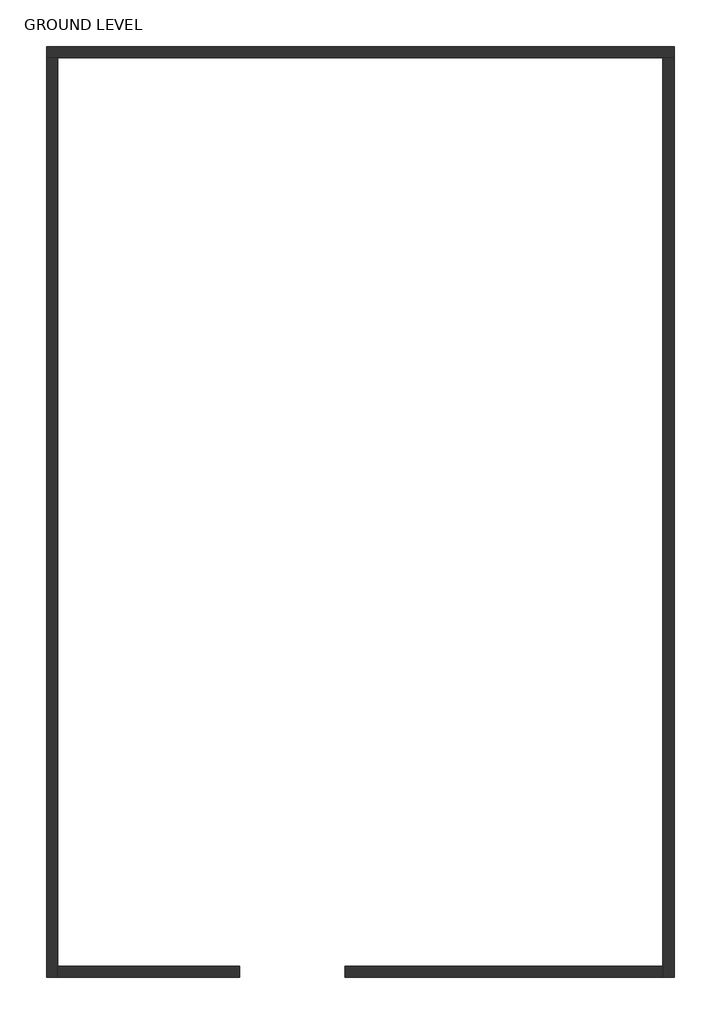
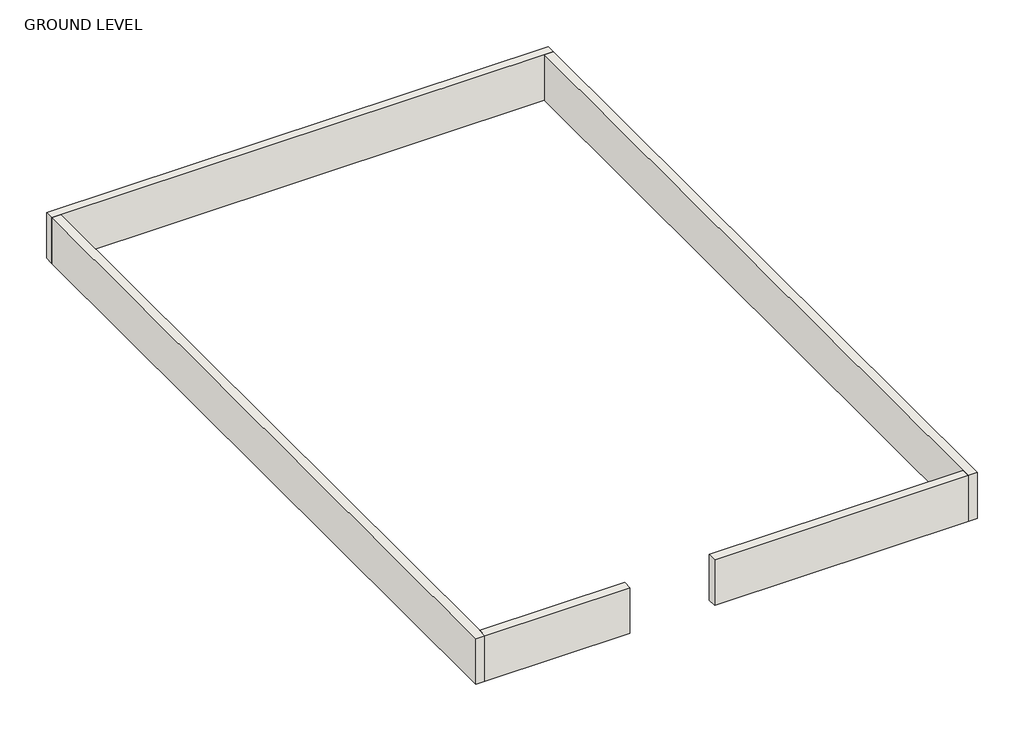
# One storey: 5 walls.
"""IFC4 building model written with IfcOpenShell, lengths in millimetres."""

from ifc_helpers import new_model, si_unit, origin, origin_with_axes, place, context, project, spatial, polyline, outline, extrude, faceted_brep, element, save

model = new_model("IFC4")

# Units and contexts
model_context = context("Model", 3, world=origin())
ifc_project = project(units=[si_unit("LENGTHUNIT", "METRE", prefix="MILLI")], contexts=[model_context])

# Site, building, storey
site = spatial("IfcSite", under=ifc_project)
building = spatial("IfcBuilding", under=site)
storey = spatial("IfcBuildingStorey", under=building, Name="GROUND LEVEL", Elevation=0.0)

# Walls
placement = place(None, origin())
element("IfcWall", 1, ObjectType="EXTERIOR WALL 9\"", at=placement, inside=storey, context=model_context, shape_type="Brep", body=[
    faceted_brep([(-19973.9229553, 9244.8839313, 0.0), (-19745.3229553, 9244.8839313, 0.0), (-7553.3229553, 9244.8839313, 0.0), (-7324.7229553, 9244.8839313, 0.0), (-7324.7229553, 9244.8839313, 1219.2), (-7553.3229553, 9244.8839313, 1219.2), (-19745.3229553, 9244.8839313, 1219.2), (-19973.9229553, 9244.8839313, 1219.2), (-19973.9229553, 9473.4839313, 0.0), (-19973.9229553, 9473.4839313, 1219.2), (-7324.7229553, 9473.4839313, 1219.2), (-7324.7229553, 9473.4839313, 0.0)], [[[0, 1, 2, 3, 4, 5, 6, 7]], [[8, 9, 10, 11]], [[3, 2, 1, 0, 8, 11]], [[7, 6, 5, 4, 10, 9]], [[4, 3, 11, 10]], [[0, 7, 9, 8]]]),
])
element("IfcWall", 2, ObjectType="EXTERIOR WALL 9\"", at=placement, inside=storey, context=model_context, shape_type="Brep", body=[
    faceted_brep([(-7553.3229553, 9244.8839313, 0.0), (-7553.3229553, -9044.7035687, 0.0), (-7553.3229553, -9273.3035687, 0.0), (-7553.3229553, -9273.3035687, 1219.2), (-7553.3229553, -9044.7035687, 1219.2), (-7553.3229553, 9244.8839313, 1219.2), (-7324.7229553, 9244.8839313, 0.0), (-7324.7229553, 9244.8839313, 1219.2), (-7324.7229553, -9273.3035687, 1219.2), (-7324.7229553, -9273.3035687, 0.0)], [[[0, 1, 2, 3, 4, 5]], [[6, 7, 8, 9]], [[2, 1, 0, 6, 9]], [[5, 4, 3, 8, 7]], [[0, 5, 7, 6]], [[3, 2, 9, 8]]]),
])
element("IfcWall", 3, ObjectType="EXTERIOR WALL 9\"", at=placement, inside=storey, context=model_context, shape_type="SweptSolid", body=[
    extrude(outline(polyline([(-13954.1229553, -9044.7035687), (-7553.3229553, -9044.7035687), (-7553.3229553, -9273.3035687), (-13954.1229553, -9273.3035687), (-13954.1229553, -9044.7035687)])), origin_with_axes(), (0.0, 0.0, 1.0), 1219.2),
])
element("IfcWall", 4, ObjectType="EXTERIOR WALL 9\"", at=placement, inside=storey, context=model_context, shape_type="Brep", body=[
    faceted_brep([(-19745.3229553, -9273.3035687, 0.0), (-19745.3229553, -9044.7035687, 0.0), (-19745.3229553, 9244.8839313, 0.0), (-19745.3229553, 9244.8839313, 1219.2), (-19745.3229553, -9044.7035687, 1219.2), (-19745.3229553, -9273.3035687, 1219.2), (-19973.9229553, -9273.3035687, 0.0), (-19973.9229553, -9273.3035687, 1219.2), (-19973.9229553, 9244.8839313, 1219.2), (-19973.9229553, 9244.8839313, 0.0)], [[[0, 1, 2, 3, 4, 5]], [[6, 7, 8, 9]], [[2, 1, 0, 6, 9]], [[5, 4, 3, 8, 7]], [[3, 2, 9, 8]], [[0, 5, 7, 6]]]),
])
element("IfcWall", 5, ObjectType="EXTERIOR WALL 9\"", at=placement, inside=storey, context=model_context, shape_type="SweptSolid", body=[
    extrude(outline(polyline([(-16087.7229553, -9273.3035687), (-19745.3229553, -9273.3035687), (-19745.3229553, -9044.7035687), (-16087.7229553, -9044.7035687), (-16087.7229553, -9273.3035687)])), origin_with_axes(), (0.0, 0.0, 1.0), 1219.2),
])

save(model, "model.ifc")

# Revit data of these elements
# Type "EXTERIOR WALL 9\""
#   Assembly Code = "B2010"
#   Layers, outside or top first: 0' - 9" "EXTERIOR WALL WHITE COLOUR" (function 1)
# Elements 1, 2, 3, 4, 5 (IfcWall, "EXTERIOR WALL 9\"")
#   Top Offset = 0' - 0"
#   Base Offset = 0' - 0"
#   Unconnected Height = 4' - 0"
#   wall height = 4' - 0"
#   Phase Created = New Construction
#   Base Constraint = GROUND LEVEL
#   Materials on its faces: "EXTERIOR WALL WHITE COLOUR"
# Materials
#   "EXTERIOR WALL WHITE COLOUR": class "Generic", colour RGB 120 120 120, transparency 0, Cost = 0
